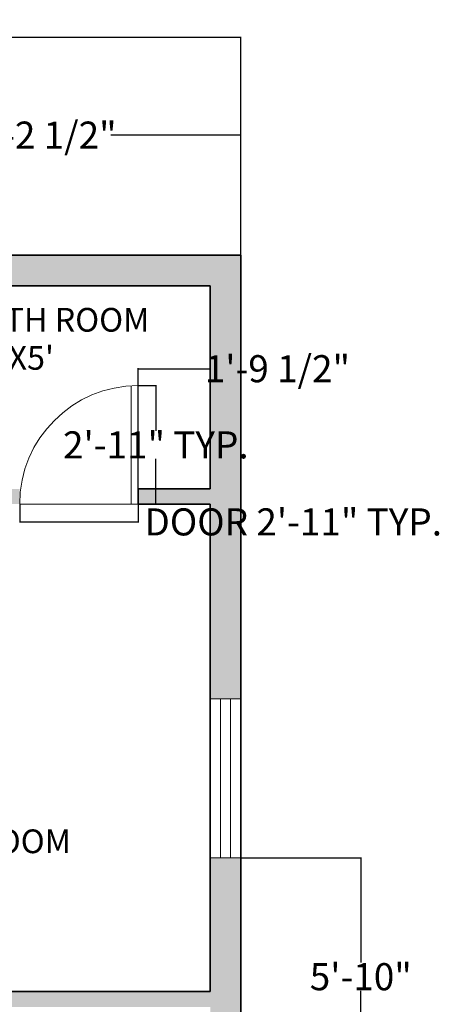
# Model space of a CAD drawing. Units: inches. Extents: x 638 to 1303, y 1 to 699.
# Tile 21 of 21: x 1163 to 1287, y 409 to 699. Entities that reach past the tile are written whole.
import ezdxf

# ---------------------------------------------------------------- set-up
doc = ezdxf.new("R2010")
doc.units = ezdxf.units.IN
doc.header["$MEASUREMENT"] = 0
for name, color, linetype, lineweight in [('A-ANNO-DIMS', 2, 'Continuous', 18), ('A-AREA-IDEN', 7, 'Continuous', 18), ('A-DOOR', 4, 'Continuous', 18), ('A-GLAZ', 4, 'Continuous', 18), ('A-WALL', 7, 'Continuous', 35)]:
    doc.layers.add(name, color=color, linetype=linetype, lineweight=lineweight)
doc.layers.add('A-WALL-PATT', color=143, linetype='Continuous', lineweight=13, true_color=0x7aafdf)
doc.styles.get("Standard").update_dxf_attribs({"font": 'arial.ttf'})
doc.dimstyles.get("Standard").update_dxf_attribs({"dimtxt": 8, "dimasz": 0.18, "dimexe": 0.18, "dimexo": 0.0625, "dimgap": 0.09, "dimtad": 0, "dimtih": 1, "dimtoh": 1, "dimdec": 4, "dimzin": 0, "dimdsep": 46, "dimlunit": 3, "dimtxsty": 'Standard', "dimcen": 0.09, "dimadec": 0, "dimazin": 0, "dimtfac": 1, "dimtdec": 4, "dimtofl": 0, "dimtmove": 0, "dimatfit": 3, "dimfxl": 1, "dimtolj": 1, "dimtzin": 0, "dimarcsym": 0})

# ---------------------------------------------------------------- blocks, each defined once
blk = doc.blocks.new('*D2')
at = {"layer": 'A-ANNO-DIMS', "color": 0, "lineweight": -2, "transparency": 16777216}
for p, q in [((697.24, 629.88), (697.24, 694.35)), ((697.42, 694.17), (934.76, 694.17)), ((1228.06, 694.17), (990.71, 694.17)), ((1228.24, 629.88), (1228.24, 694.35))]:
    blk.add_line(p, q, dxfattribs=at)
at = {"layer": 'A-ANNO-DIMS', "color": 0, "transparency": 16777216}
for points in [[(697.42, 694.2), (697.42, 694.14), (697.24, 694.17)], [(1228.06, 694.2), (1228.06, 694.14), (1228.24, 694.17)]]:
    blk.add_solid(points, dxfattribs=at)
at = {"layer": 'Defpoints', "color": 0, "transparency": 16777216}
for p in [(1228.24, 694.17), (697.24, 629.82), (1228.24, 629.82)]:
    blk.add_point(p, dxfattribs=at)
at = {"layer": 'A-ANNO-DIMS', "color": 0, "transparency": 16777216, "insert": (962.74, 694.17), "char_height": 8, "attachment_point": 5}
blk.add_mtext('\\A1;44\'-3.0000"', dxfattribs=at)
blk = doc.blocks.new('DOOR-SWING-35')
for p, q in [((33, 0), (33, 34.94)), ((35, 0), (35, 35)), ((0, 0), (35, 0))]:
    blk.add_line(p, q)
blk.add_arc((35, 0), 35, 90, 180)
blk = doc.blocks.new('WIN-47')
for p, q in [((47, 9), (0, 9)), ((0, 9), (0, 0)), ((47, 0), (47, 9)), ((0, 6), (47, 6)), ((0, 3), (47, 3)), ((0, 0), (47, 0))]:
    blk.add_line(p, q)
blk = doc.blocks.new('*D28')
at = {"layer": 'A-ANNO-DIMS', "color": 0, "lineweight": -2, "transparency": 16777216}
for p, q in [((1162.9, 556.26), (1162.9, 550.89)), ((1197.9, 556.26), (1197.9, 550.89)), ((1163.08, 551.07), (1197.72, 551.07)), ((1197.9, 551.07), (1198.08, 551.07))]:
    blk.add_line(p, q, dxfattribs=at)
at = {"layer": 'A-ANNO-DIMS', "color": 0, "transparency": 16777216}
for points in [[(1163.08, 551.1), (1163.08, 551.04), (1162.9, 551.07)], [(1197.72, 551.1), (1197.72, 551.04), (1197.9, 551.07)]]:
    blk.add_solid(points, dxfattribs=at)
at = {"layer": 'Defpoints', "color": 0, "transparency": 16777216}
for p in [(1162.9, 556.32), (1197.9, 556.32), (1197.9, 551.07)]:
    blk.add_point(p, dxfattribs=at)
at = {"layer": 'A-ANNO-DIMS', "color": 0, "transparency": 16777216, "insert": (1243.77, 551.07), "char_height": 8, "attachment_point": 5}
blk.add_mtext('\\A1;DOOR 2\'-11" TYP.', dxfattribs=at)
blk = doc.blocks.new('*D29')
at = {"layer": 'A-ANNO-DIMS', "color": 0, "lineweight": -2, "transparency": 16777216}
for p, q in [((1197.96, 591.32), (1203.33, 591.32)), ((1203.15, 591.14), (1203.15, 577.93)), ((1203.15, 556.5), (1203.15, 569.71)), ((1197.96, 556.32), (1203.33, 556.32))]:
    blk.add_line(p, q, dxfattribs=at)
at = {"layer": 'A-ANNO-DIMS', "color": 0, "transparency": 16777216}
for points in [[(1203.12, 591.14), (1203.18, 591.14), (1203.15, 591.32)], [(1203.12, 556.5), (1203.18, 556.5), (1203.15, 556.32)]]:
    blk.add_solid(points, dxfattribs=at)
at = {"layer": 'Defpoints', "color": 0, "transparency": 16777216}
for p in [(1197.9, 591.32), (1203.15, 591.32), (1197.9, 556.32)]:
    blk.add_point(p, dxfattribs=at)
at = {"layer": 'A-ANNO-DIMS', "color": 0, "transparency": 16777216, "insert": (1203.15, 573.82), "char_height": 8, "attachment_point": 5}
blk.add_mtext('\\A1;2\'-11" TYP.', dxfattribs=at)
blk = doc.blocks.new('*D50')
at = {"layer": 'A-ANNO-DIMS', "color": 0, "lineweight": -2, "transparency": 16777216}
for p, q in [((1228.3, 451.8), (1263.92, 451.8)), ((1263.74, 451.62), (1263.74, 420.91)), ((1263.74, 381.84), (1263.74, 412.56)), ((1228.3, 381.66), (1263.92, 381.66))]:
    blk.add_line(p, q, dxfattribs=at)
at = {"layer": 'A-ANNO-DIMS', "color": 0, "transparency": 16777216}
for points in [[(1263.71, 451.62), (1263.77, 451.62), (1263.74, 451.8)], [(1263.71, 381.84), (1263.77, 381.84), (1263.74, 381.66)]]:
    blk.add_solid(points, dxfattribs=at)
at = {"layer": 'Defpoints', "color": 0, "transparency": 16777216}
for p in [(1228.24, 451.8), (1263.74, 451.8), (1228.24, 381.66)]:
    blk.add_point(p, dxfattribs=at)
at = {"layer": 'A-ANNO-DIMS', "color": 0, "transparency": 16777216, "insert": (1263.74, 416.73), "char_height": 8, "attachment_point": 5}
blk.add_mtext('\\A1;5\'-10"', dxfattribs=at)
blk = doc.blocks.new('*D54')
at = {"layer": 'A-ANNO-DIMS', "color": 0, "lineweight": -2, "transparency": 16777216}
for p, q in [((1105.85, 629.88), (1105.85, 665.5)), ((1106.03, 665.32), (1144.27, 665.32)), ((1228.06, 665.32), (1189.82, 665.32)), ((1228.24, 629.88), (1228.24, 665.5))]:
    blk.add_line(p, q, dxfattribs=at)
at = {"layer": 'A-ANNO-DIMS', "color": 0, "transparency": 16777216}
for points in [[(1106.03, 665.35), (1106.03, 665.29), (1105.85, 665.32)], [(1228.06, 665.35), (1228.06, 665.29), (1228.24, 665.32)]]:
    blk.add_solid(points, dxfattribs=at)
at = {"layer": 'Defpoints', "color": 0, "transparency": 16777216}
for p in [(1228.24, 665.32), (1105.85, 629.82), (1228.24, 629.82)]:
    blk.add_point(p, dxfattribs=at)
at = {"layer": 'A-ANNO-DIMS', "color": 0, "transparency": 16777216, "insert": (1167.05, 665.32), "char_height": 8, "attachment_point": 5}
blk.add_mtext('\\A1;10\'-2 1/2"', dxfattribs=at)
blk = doc.blocks.new('*D69')
at = {"layer": 'A-ANNO-DIMS', "color": 0, "lineweight": -2, "transparency": 16777216}
for p, q in [((1197.9, 560.88), (1197.9, 596.5)), ((1198.08, 596.32), (1219.06, 596.32)), ((1219.24, 560.88), (1219.24, 596.5)), ((1219.24, 596.32), (1219.42, 596.32))]:
    blk.add_line(p, q, dxfattribs=at)
at = {"layer": 'A-ANNO-DIMS', "color": 0, "transparency": 16777216}
for points in [[(1198.08, 596.35), (1198.08, 596.29), (1197.9, 596.32)], [(1219.06, 596.35), (1219.06, 596.29), (1219.24, 596.32)]]:
    blk.add_solid(points, dxfattribs=at)
at = {"layer": 'Defpoints', "color": 0, "transparency": 16777216}
for p in [(1219.24, 596.32), (1197.9, 560.82), (1219.24, 560.82)]:
    blk.add_point(p, dxfattribs=at)
at = {"layer": 'A-ANNO-DIMS', "color": 0, "transparency": 16777216, "insert": (1239.09, 596.32), "char_height": 8, "attachment_point": 5}
blk.add_mtext('\\A1;1\'-9 1/2"', dxfattribs=at)

msp = doc.modelspace()

# ---------------------------------------------------------------- hatches: boundary and pattern name
at = {"layer": 'A-WALL-PATT'}
h = msp.add_hatch(color=256, dxfattribs=at)
h.dxf.hatch_style = 1
h.paths.add_polyline_path([(973.34524, 629.81895), (793.35541, 629.81895), (793.35541, 620.81895), (850.23798, 620.81895), (922.23798, 620.81895), (922.23798, 524.81895), (908.94335, 524.81895), (908.94335, 520.31895), (926.73798, 520.31895), (926.73798, 544.31895), (979.3571, 544.31895), (979.3571, 548.81895), (926.73798, 548.81895), (926.73798, 620.81895), (973.34524, 620.81895)])
h.paths.add_polyline_path([(758.35541, 629.81895), (697.23798, 629.81895), (697.23798, 586.77451), (706.23798, 586.77451), (706.23798, 620.81895), (758.35541, 620.81895)])
h.paths.add_polyline_path([(1075.85281, 629.81895), (1003.34524, 629.81895), (1003.34524, 620.81895), (1046.73798, 620.81895), (1046.73798, 560.81895), (1046.73798, 548.81895), (1026.3571, 548.81895), (1026.3571, 544.31895), (1046.73798, 544.31895), (1046.73798, 486.87457), (1051.23798, 486.87457), (1051.23798, 556.31895), (1162.89753, 556.31895), (1162.89753, 560.81895), (1051.23798, 560.81895), (1051.23798, 620.81895), (1075.85281, 620.81895)])
h.paths.add_polyline_path([(1228.23798, 629.81895), (1105.85281, 629.81895), (1105.85281, 620.81895), (1219.23798, 620.81895), (1219.23798, 560.81895), (1197.89753, 560.81895), (1197.89753, 556.31895), (1219.23798, 556.31895), (1219.23798, 498.80084), (1228.23798, 498.80084)])
h.paths.add_polyline_path([(1051.23798, 439.87457), (1046.73798, 439.87457), (1046.73798, 407.81895), (1219.23798, 407.81895), (1219.23798, 381.66175), (1228.23798, 381.66175), (1228.23798, 451.80084), (1219.23798, 451.80084), (1219.23798, 412.31895), (1051.23798, 412.31895)])
h.paths.add_polyline_path([(1228.23798, 346.66175), (1219.23798, 346.66175), (1219.23798, 335.81895), (1046.73798, 335.81895), (1046.73798, 273.56895), (1051.23798, 273.56895), (1051.23798, 331.31895), (1219.23798, 331.31895), (1219.23798, 308.99654), (1228.23798, 308.99654)])
h.paths.add_polyline_path([(1228.23798, 261.99654), (1219.23798, 261.99654), (1219.23798, 211.31895), (1051.23798, 211.31895), (1051.23798, 226.56895), (1046.73798, 226.56895), (1046.73798, 211.31895), (983.84714, 211.31895), (983.84714, 206.81895), (1219.23798, 206.81895), (1219.23798, 166.83987), (1228.23798, 166.83987)])
h.paths.add_polyline_path([(1228.23798, 119.83987), (1219.23798, 119.83987), (1219.23798, 50.81895), (1197.89277, 50.81895), (1197.89277, 41.81895), (1228.23798, 41.81895)])
h.paths.add_polyline_path([(1162.89277, 50.81895), (1069.02949, 50.81895), (1069.02949, 41.81895), (1162.89277, 41.81895)])
h.paths.add_polyline_path([(1010.02949, 50.81895), (941.89631, 50.81895), (917.77455, 50.81895), (917.77455, 41.81895), (941.89631, 41.81895), (1010.02949, 41.81895)])
h.paths.add_polyline_path([(882.77455, 50.81895), (854.73798, 50.81895), (854.73798, 145.50379), (850.23798, 145.50379), (850.23798, 50.81895), (793.49755, 50.81895), (793.49755, 41.81895), (882.77455, 41.81895)])
h.paths.add_polyline_path([(746.49755, 50.81895), (706.23798, 50.81895), (706.23798, 96.57416), (697.23798, 96.57416), (697.23798, 41.81895), (746.49755, 41.81895)])
h.paths.add_polyline_path([(706.23798, 206.81895), (714.01165, 206.81895), (714.01165, 211.31895), (706.23798, 211.31895), (706.23798, 251.21966), (697.23798, 251.21966), (697.23798, 143.57416), (706.23798, 143.57416)])
h.paths.add_polyline_path([(923.84714, 211.31895), (854.73798, 211.31895), (854.73798, 397.8313), (850.23798, 397.8313), (850.23798, 388.31895), (747.9539, 388.31895), (747.9539, 383.81895), (850.23798, 383.81895), (850.23798, 311.81895), (706.23798, 311.81895), (706.23798, 342.78787), (697.23798, 342.78787), (697.23798, 281.21966), (706.23798, 281.21966), (706.23798, 307.31895), (850.23798, 307.31895), (850.23798, 211.31895), (749.01165, 211.31895), (749.01165, 206.81895), (850.23798, 206.81895), (850.23798, 192.50379), (854.73798, 192.50379), (854.73798, 206.81895), (923.84714, 206.81895)])
h.paths.add_polyline_path([(706.23798, 434.70471), (697.23798, 434.70471), (697.23798, 372.78787), (706.23798, 372.78787), (706.23798, 383.81895), (712.9539, 383.81895), (712.9539, 388.31895), (706.23798, 388.31895)])
h.paths.add_polyline_path([(706.23798, 520.31895), (850.23798, 520.31895), (850.23798, 444.8313), (854.73798, 444.8313), (854.73798, 520.31895), (861.94335, 520.31895), (861.94335, 524.81895), (706.23798, 524.81895), (706.23798, 551.77451), (697.23798, 551.77451), (697.23798, 481.70471), (706.23798, 481.70471)])

# ---------------------------------------------------------------- linework, layer by layer
at = {"layer": 'A-WALL'}
for p, q in [((1228.23798, 629.81895), (697.23798, 629.81895)), ((1228.23798, 629.81895), (1228.23798, 41.81895)), ((1219.23798, 620.81895), (1051.23798, 620.81895)), ((1219.23798, 620.81895), (1219.23798, 560.81895)), ((1219.23798, 560.81895), (1197.89753, 560.81895)), ((1197.89753, 560.81895), (1197.89753, 556.31895)), ((1219.23798, 556.31895), (1197.89753, 556.31895)), ((1219.23798, 556.31895), (1219.23798, 412.31895)), ((1219.23798, 412.31895), (1051.23798, 412.31895))]:
    msp.add_line(p, q, dxfattribs=at)

# ---------------------------------------------------------------- block references
at = {"layer": 'A-DOOR'}
msp.add_blockref('DOOR-SWING-35', (1162.898, 556.319), dxfattribs=at)
at = {"layer": 'A-GLAZ', "rotation": 270.0000000000011}
msp.add_blockref('WIN-47', (1219.23803, 498.80039), dxfattribs=at)

# ---------------------------------------------------------------- texts
at = {"layer": 'A-AREA-IDEN'}
for s, p in [('BATH ROOM', (1146.35423, 607.27456)), ("14'X5'", (1146.35423, 596.02968)), ('BED ROOM', (1129.45331, 453.22006))]:
    msp.add_text(s, height=7, dxfattribs=at).set_placement(p)

# ---------------------------------------------------------------- dimensions: what is measured, and where the dimension line sits
at = {"layer": 'A-ANNO-DIMS'}
for base, p1, p2, override, picture, middle in [((1228.23798, 694.16557), (697.23798, 629.81895), (1228.23798, 629.81895), {"dimclrd": 0, "dimclre": 0, "dimclrt": 0}, '*D2', (962.73798, 694.16557)), ((1228.23798, 665.31895), (1105.85281, 629.81895), (1228.23798, 629.81895), {"dimdec": 1, "dimlfac": 1, "dimrnd": 0, "dimzin": 1, "dimdsep": 46, "dimlunit": 4, "dimfrac": 2}, '*D54', (1167.0454, 665.31895)), ((1219.23798, 596.31895), (1197.89753, 560.81895), (1219.23798, 560.81895), {"dimdec": 1, "dimlfac": 1, "dimrnd": 0, "dimzin": 1, "dimdsep": 46, "dimlunit": 4, "dimfrac": 2}, '*D69', (1239.08506, 596.31895))]:
    dim = msp.add_linear_dim(base=base, p1=p1, p2=p2, dimstyle='Standard', override=override, dxfattribs=at)
    dim.commit()
    dim.dimension.update_dxf_attribs({"geometry": picture, "text_midpoint": middle})
dim = msp.add_linear_dim(base=(1203.14753, 591.31895), p1=(1197.89753, 556.31895), p2=(1197.89753, 591.31895), angle=90, text='<> TYP.', dimstyle='Standard', override={"dimdec": 1, "dimlfac": 1, "dimrnd": 0, "dimzin": 1, "dimdsep": 46, "dimlunit": 4, "dimfrac": 2}, dxfattribs=at)
dim.commit()
dim.dimension.update_dxf_attribs({"geometry": '*D29', "text_midpoint": (1203.14753, 573.81895)})
dim = msp.add_linear_dim(base=(1197.89753, 551.06895), p1=(1162.89753, 556.31895), p2=(1197.89753, 556.31895), text='DOOR <> TYP.', dimstyle='Standard', override={"dimdec": 1, "dimlfac": 1, "dimrnd": 0, "dimzin": 1, "dimdsep": 46, "dimlunit": 4, "dimfrac": 2}, dxfattribs=at)
dim.commit()
dim.dimension.update_dxf_attribs({"geometry": '*D28', "text_midpoint": (1243.77462, 551.06895)})
dim = msp.add_linear_dim(base=(1263.73798, 451.80084), p1=(1228.23798, 381.66175), p2=(1228.23798, 451.80084), angle=90, dimstyle='Standard', override={"dimdec": 1, "dimlfac": 1, "dimrnd": 0, "dimzin": 1, "dimdsep": 46, "dimlunit": 4, "dimfrac": 2}, dxfattribs=at)
dim.commit()
dim.dimension.update_dxf_attribs({"geometry": '*D50', "text_midpoint": (1263.73798, 416.7313)})

doc.saveas('drawing.dxf')
